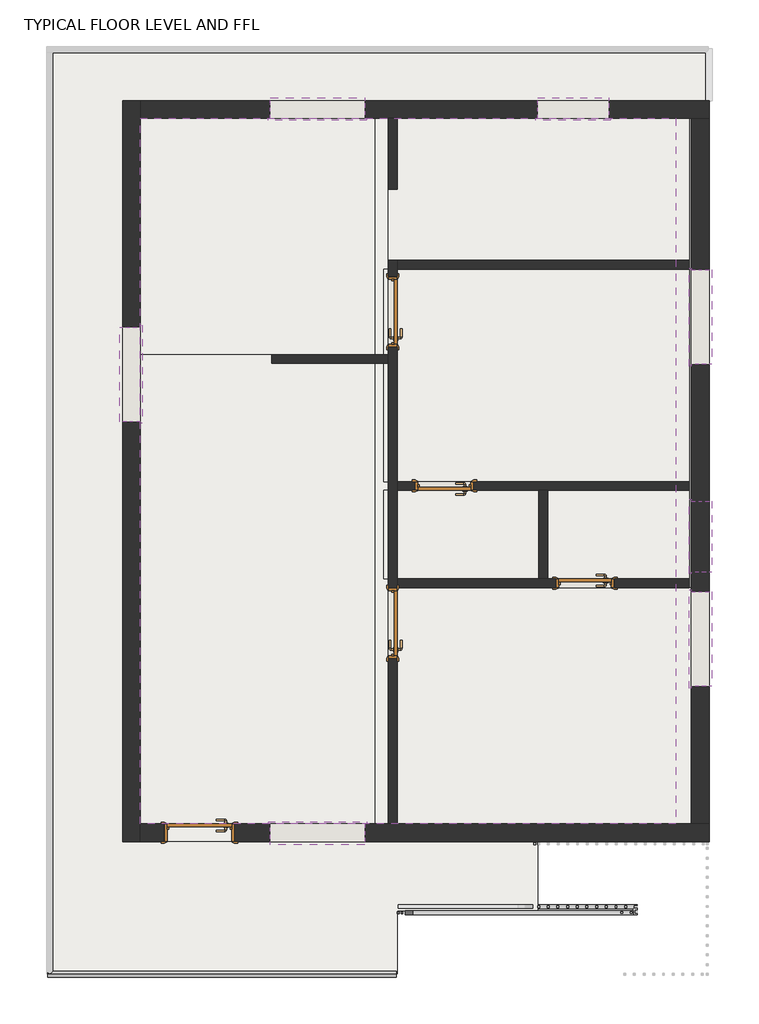
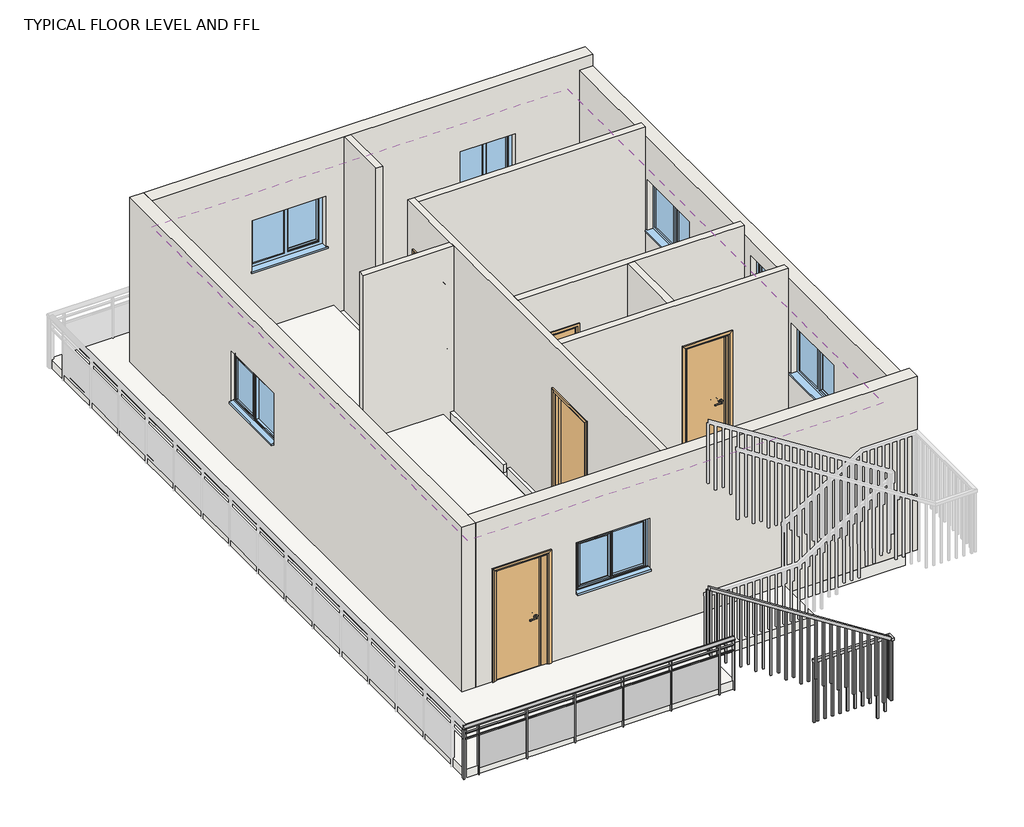
# One storey, part 1 of 3: 11 walls, 9 slabs, 7 windows, 5 doors, 2 railings, 1 covering.
"""IFC4 building model written with IfcOpenShell, lengths in millimetres."""

from ifc_helpers import new_model, si_unit, point, frame, origin, place, context, project, spatial, polyline, ellipse_curve, trimmed, outline, extrude, faceted_brep, transform, mapped, element, save
from ifc_brep_helpers import plane_surface, extruded_surface, advanced_brep
from components import doors_intsgl_d1_d2de26da, doors_intsgl_d1_5aeab8eb, doors_intsgl_d2_21b53886, doors_intsgl_d2_1f5f3f16, windows_dbl_plain_w1_9e0d93ab, windows_dbl_plain_w2_c69f14ef, windows_sgl_plain_v_28d0678b

model = new_model("IFC4")

# Units and contexts
model_context = context("Model", 3, world=origin())
ifc_project = project(units=[si_unit("LENGTHUNIT", "METRE", prefix="MILLI")], contexts=[model_context])

# Site, building, storey
site = spatial("IfcSite", under=ifc_project)
building = spatial("IfcBuilding", under=site)
storey = spatial("IfcBuildingStorey", under=building, Name="TYPICAL FLOOR LEVEL AND FFL", Elevation=3535.68)

# Covering
placement = place(None, origin())
element("IfcCovering", 1, at=placement, inside=storey, context=model_context, shape_type="SweptSolid", body=[
    extrude(outline(polyline([(-6897.0620435, -885.5593981), (-6897.0620435, -9991.0521308), (-10668.9827978, -9991.0521308), (-13810.6009005, -9991.0521308), (-13810.6009005, -885.5593981), (-6897.0620435, -885.5593981)])), frame((0.0, 0.0, 6126.48), z_axis=(0.0, 0.0, 1.0), x_axis=(1.0, 0.0, 0.0)), (0.0, 0.0, 1.0), 57.0),
])

# Doors
doors_intsgl_d1_shape = doors_intsgl_d1_d2de26da(model_context)
element("IfcDoor", 2, ObjectType="Doors_IntSgl : D1", at=placement, inside=storey, context=model_context, shape_type="MappedRepresentation", body=[
    mapped(doors_intsgl_d1_shape, transform((-10553.0840108, -7400.866169, 3685.6416), x_axis=(0.0, 1.0, 0.0), y_axis=(-1.0, 0.0, 0.0), z_axis=(0.0, 0.0, 1.0))),
])
element("IfcDoor", 3, ObjectType="Doors_IntSgl : D1", at=placement, inside=storey, context=model_context, shape_type="MappedRepresentation", body=[
    mapped(doors_intsgl_d1_shape, transform((-10553.0840108, -3381.2262014, 3685.6416), x_axis=(0.0, 1.0, 0.0), y_axis=(-1.0, 0.0, 0.0), z_axis=(0.0, 0.0, 1.0))),
])
doors_intsgl_d1_2_shape = doors_intsgl_d1_5aeab8eb(model_context)
element("IfcDoor", 4, ObjectType="Doors_IntSgl : D1", at=placement, inside=storey, context=model_context, shape_type="MappedRepresentation", body=[
    mapped(doors_intsgl_d1_2_shape, transform((-13048.4335145, -10105.3521308, 3535.68), x_axis=(-1.0, 0.0, 0.0), y_axis=(0.0, -1.0, 0.0), z_axis=(0.0, 0.0, 1.0))),
])
doors_intsgl_d2_shape = doors_intsgl_d2_21b53886(model_context)
element("IfcDoor", 5, ObjectType="Doors_IntSgl : D2", at=placement, inside=storey, context=model_context, shape_type="MappedRepresentation", body=[
    mapped(doors_intsgl_d2_shape, transform((-9886.3340108, -5628.9784114, 3685.6416), x_axis=(-1.0, 0.0, 0.0), y_axis=(0.0, -1.0, 0.0), z_axis=(0.0, 0.0, 1.0))),
])
doors_intsgl_d2_2_shape = doors_intsgl_d2_1f5f3f16(model_context)
element("IfcDoor", 6, ObjectType="Doors_IntSgl : D2", at=placement, inside=storey, context=model_context, shape_type="MappedRepresentation", body=[
    mapped(doors_intsgl_d2_2_shape, transform((-8070.4366309, -6886.516169, 3685.6416), x_axis=(-1.0, 0.0, 0.0), y_axis=(0.0, -1.0, 0.0), z_axis=(0.0, 0.0, 1.0))),
])

# Railings
element("IfcRailing", 7, ObjectType="1100mm", at=placement, inside=storey, context=model_context, shape_type="SolidModel", body=[
    faceted_brep([(-10457.8773536, -11114.0601959, 4838.88), (-10457.8773536, -11114.0601959, 4779.5164137), (-10457.8773536, -11164.0601959, 4779.5164137), (-10457.8773536, -11164.0601959, 4838.88), (-7447.5340108, -11114.0601959, 2912.2269781), (-7447.5340108, -11164.0601959, 2912.2269781), (-7447.5340108, -11164.0601959, 2852.8633918), (-7447.5340108, -11114.0601959, 2852.8633918)], [[[0, 1, 2, 3]], [[4, 5, 6, 7]], [[1, 0, 4, 7]], [[2, 1, 7, 6]], [[3, 2, 6, 5]], [[0, 3, 5, 4]]]),
    faceted_brep([(-7447.5340108, -11164.0601959, 2888.16), (-7447.5340108, -11164.0601959, 2838.16), (-7397.5340108, -11164.0601959, 2838.16), (-7397.5340108, -11164.0601959, 2888.16), (-7447.5340108, -11083.3255223, 2888.16), (-7447.5340108, -11083.3255223, 2838.16), (-7397.5340108, -11033.3255223, 2838.16), (-7397.5340108, -11033.3255223, 2888.16), (-8680.149573, -11083.3255223, 2888.16), (-8680.149573, -11033.3255223, 2888.16), (-8680.149573, -11033.3255223, 2838.16), (-8680.149573, -11083.3255223, 2838.16)], [[[0, 1, 2, 3]], [[1, 0, 4, 5]], [[2, 1, 5, 6]], [[3, 2, 6, 7]], [[0, 3, 7, 4]], [[8, 9, 10, 11]], [[5, 4, 8, 11]], [[6, 5, 11, 10]], [[7, 6, 10, 9]], [[4, 7, 9, 8]]]),
    extrude(outline(polyline([(-8597.5340108, -11045.8255223), (-8597.5340108, -11070.8255223), (-8622.5340108, -11070.8255223), (-8622.5340108, -11045.8255223), (-8597.5340108, -11045.8255223)])), frame((0.0, 0.0, 1788.16), z_axis=(0.0, 0.0, 1.0), x_axis=(1.0, 0.0, 0.0)), (0.0, 0.0, 1.0), 1050.0),
    extrude(outline(polyline([(-8472.5340108, -11045.8255223), (-8472.5340108, -11070.8255223), (-8497.5340108, -11070.8255223), (-8497.5340108, -11045.8255223), (-8472.5340108, -11045.8255223)])), frame((0.0, 0.0, 1788.16), z_axis=(0.0, 0.0, 1.0), x_axis=(1.0, 0.0, 0.0)), (0.0, 0.0, 1.0), 1050.0),
    extrude(outline(polyline([(-8347.5340108, -11045.8255223), (-8347.5340108, -11070.8255223), (-8372.5340108, -11070.8255223), (-8372.5340108, -11045.8255223), (-8347.5340108, -11045.8255223)])), frame((0.0, 0.0, 1788.16), z_axis=(0.0, 0.0, 1.0), x_axis=(1.0, 0.0, 0.0)), (0.0, 0.0, 1.0), 1050.0),
    extrude(outline(polyline([(-8222.5340108, -11045.8255223), (-8222.5340108, -11070.8255223), (-8247.5340108, -11070.8255223), (-8247.5340108, -11045.8255223), (-8222.5340108, -11045.8255223)])), frame((0.0, 0.0, 1788.16), z_axis=(0.0, 0.0, 1.0), x_axis=(1.0, 0.0, 0.0)), (0.0, 0.0, 1.0), 1050.0),
    extrude(outline(polyline([(-8097.5340108, -11045.8255223), (-8097.5340108, -11070.8255223), (-8122.5340108, -11070.8255223), (-8122.5340108, -11045.8255223), (-8097.5340108, -11045.8255223)])), frame((0.0, 0.0, 1788.16), z_axis=(0.0, 0.0, 1.0), x_axis=(1.0, 0.0, 0.0)), (0.0, 0.0, 1.0), 1050.0),
    extrude(outline(polyline([(-7972.5340108, -11045.8255223), (-7972.5340108, -11070.8255223), (-7997.5340108, -11070.8255223), (-7997.5340108, -11045.8255223), (-7972.5340108, -11045.8255223)])), frame((0.0, 0.0, 1788.16), z_axis=(0.0, 0.0, 1.0), x_axis=(1.0, 0.0, 0.0)), (0.0, 0.0, 1.0), 1050.0),
    extrude(outline(polyline([(-7847.5340108, -11045.8255223), (-7847.5340108, -11070.8255223), (-7872.5340108, -11070.8255223), (-7872.5340108, -11045.8255223), (-7847.5340108, -11045.8255223)])), frame((0.0, 0.0, 1788.16), z_axis=(0.0, 0.0, 1.0), x_axis=(1.0, 0.0, 0.0)), (0.0, 0.0, 1.0), 1050.0),
    extrude(outline(polyline([(-7722.5340108, -11045.8255223), (-7722.5340108, -11070.8255223), (-7747.5340108, -11070.8255223), (-7747.5340108, -11045.8255223), (-7722.5340108, -11045.8255223)])), frame((0.0, 0.0, 1788.16), z_axis=(0.0, 0.0, 1.0), x_axis=(1.0, 0.0, 0.0)), (0.0, 0.0, 1.0), 1050.0),
    extrude(outline(polyline([(-7597.5340108, -11045.8255223), (-7597.5340108, -11070.8255223), (-7622.5340108, -11070.8255223), (-7622.5340108, -11045.8255223), (-7597.5340108, -11045.8255223)])), frame((0.0, 0.0, 1484.4784954), z_axis=(0.0, 0.0, 1.0), x_axis=(1.0, 0.0, 0.0)), (0.0, 0.0, 1.0), 1353.6815046),
    extrude(outline(polyline([(-7472.5340108, -11045.8255223), (-7472.5340108, -11070.8255223), (-7497.5340108, -11070.8255223), (-7497.5340108, -11045.8255223), (-7472.5340108, -11045.8255223)])), frame((0.0, 0.0, 1564.4608651), z_axis=(0.0, 0.0, 1.0), x_axis=(1.0, 0.0, 0.0)), (0.0, 0.0, 1.0), 1273.6991349),
    extrude(outline(polyline([(-7410.0340108, -11089.0601959), (-7435.0340108, -11089.0601959), (-7435.0340108, -11064.0601959), (-7410.0340108, -11064.0601959), (-7410.0340108, -11089.0601959)])), frame((0.0, 0.0, 1770.6), z_axis=(0.0, 0.0, 1.0), x_axis=(1.0, 0.0, 0.0)), (0.0, 0.0, 1.0), 1067.56),
    extrude(outline(polyline([(2851.8393741, -7445.9340108), (1788.16, -7445.9340108), (1788.16, -7420.9340108), (2835.8390977, -7420.9340108), (2851.8393741, -7445.9340108)])), frame((0.0, -11151.5601959, 0.0), z_axis=(0.0, 1.0, 0.0), x_axis=(0.0, 0.0, 1.0)), (0.0, 0.0, 1.0), 25.0),
    extrude(outline(polyline([(2931.8407561, -7570.9340108), (1788.16, -7570.9340108), (1788.16, -7545.9340108), (2915.8404797, -7545.9340108), (2931.8407561, -7570.9340108)])), frame((0.0, -11151.5601959, 0.0), z_axis=(0.0, 1.0, 0.0), x_axis=(0.0, 0.0, 1.0)), (0.0, 0.0, 1.0), 25.0),
    extrude(outline(polyline([(3011.8421381, -7695.9340108), (1950.72, -7695.9340108), (1950.72, -7670.9340108), (2995.8418617, -7670.9340108), (3011.8421381, -7695.9340108)])), frame((0.0, -11151.5601959, 0.0), z_axis=(0.0, 1.0, 0.0), x_axis=(0.0, 0.0, 1.0)), (0.0, 0.0, 1.0), 25.0),
    extrude(outline(polyline([(3091.8435201, -7820.9340108), (1950.72, -7820.9340108), (1950.72, -7795.9340108), (3075.8432437, -7795.9340108), (3091.8435201, -7820.9340108)])), frame((0.0, -11151.5601959, 0.0), z_axis=(0.0, 1.0, 0.0), x_axis=(0.0, 0.0, 1.0)), (0.0, 0.0, 1.0), 25.0),
    extrude(outline(polyline([(3171.8449021, -7945.9340108), (2113.28, -7945.9340108), (2113.28, -7920.9340108), (3155.8446257, -7920.9340108), (3171.8449021, -7945.9340108)])), frame((0.0, -11151.5601959, 0.0), z_axis=(0.0, 1.0, 0.0), x_axis=(0.0, 0.0, 1.0)), (0.0, 0.0, 1.0), 25.0),
    extrude(outline(polyline([(3251.8462841, -8070.9340108), (2113.28, -8070.9340108), (2113.28, -8045.9340108), (3235.8460077, -8045.9340108), (3251.8462841, -8070.9340108)])), frame((0.0, -11151.5601959, 0.0), z_axis=(0.0, 1.0, 0.0), x_axis=(0.0, 0.0, 1.0)), (0.0, 0.0, 1.0), 25.0),
    extrude(outline(polyline([(3331.8476661, -8195.9340108), (2275.84, -8195.9340108), (2275.84, -8170.9340108), (3315.8473897, -8170.9340108), (3331.8476661, -8195.9340108)])), frame((0.0, -11151.5601959, 0.0), z_axis=(0.0, 1.0, 0.0), x_axis=(0.0, 0.0, 1.0)), (0.0, 0.0, 1.0), 25.0),
    extrude(outline(polyline([(3411.8490481, -8320.9340108), (2275.84, -8320.9340108), (2275.84, -8295.9340108), (3395.8487717, -8295.9340108), (3411.8490481, -8320.9340108)])), frame((0.0, -11151.5601959, 0.0), z_axis=(0.0, 1.0, 0.0), x_axis=(0.0, 0.0, 1.0)), (0.0, 0.0, 1.0), 25.0),
    extrude(outline(polyline([(3491.8504301, -8445.9340108), (2438.4, -8445.9340108), (2438.4, -8420.9340108), (3475.8501537, -8420.9340108), (3491.8504301, -8445.9340108)])), frame((0.0, -11151.5601959, 0.0), z_axis=(0.0, 1.0, 0.0), x_axis=(0.0, 0.0, 1.0)), (0.0, 0.0, 1.0), 25.0),
    extrude(outline(polyline([(3571.8518121, -8570.9340108), (2438.4, -8570.9340108), (2438.4, -8545.9340108), (3555.8515357, -8545.9340108), (3571.8518121, -8570.9340108)])), frame((0.0, -11151.5601959, 0.0), z_axis=(0.0, 1.0, 0.0), x_axis=(0.0, 0.0, 1.0)), (0.0, 0.0, 1.0), 25.0),
    extrude(outline(polyline([(3651.8531942, -8695.9340108), (2600.96, -8695.9340108), (2600.96, -8670.9340108), (3635.8529178, -8670.9340108), (3651.8531942, -8695.9340108)])), frame((0.0, -11151.5601959, 0.0), z_axis=(0.0, 1.0, 0.0), x_axis=(0.0, 0.0, 1.0)), (0.0, 0.0, 1.0), 25.0),
    extrude(outline(polyline([(3731.8545762, -8820.9340108), (2600.96, -8820.9340108), (2600.96, -8795.9340108), (3715.8542998, -8795.9340108), (3731.8545762, -8820.9340108)])), frame((0.0, -11151.5601959, 0.0), z_axis=(0.0, 1.0, 0.0), x_axis=(0.0, 0.0, 1.0)), (0.0, 0.0, 1.0), 25.0),
    extrude(outline(polyline([(3811.8559582, -8945.9340108), (2600.96, -8945.9340108), (2600.96, -8920.9340108), (3795.8556818, -8920.9340108), (3811.8559582, -8945.9340108)])), frame((0.0, -11151.5601959, 0.0), z_axis=(0.0, 1.0, 0.0), x_axis=(0.0, 0.0, 1.0)), (0.0, 0.0, 1.0), 25.0),
    extrude(outline(polyline([(3891.8573402, -9070.9340108), (2763.52, -9070.9340108), (2763.52, -9045.9340108), (3875.8570638, -9045.9340108), (3891.8573402, -9070.9340108)])), frame((0.0, -11151.5601959, 0.0), z_axis=(0.0, 1.0, 0.0), x_axis=(0.0, 0.0, 1.0)), (0.0, 0.0, 1.0), 25.0),
    extrude(outline(polyline([(3971.8587222, -9195.9340108), (2763.52, -9195.9340108), (2763.52, -9170.9340108), (3955.8584458, -9170.9340108), (3971.8587222, -9195.9340108)])), frame((0.0, -11151.5601959, 0.0), z_axis=(0.0, 1.0, 0.0), x_axis=(0.0, 0.0, 1.0)), (0.0, 0.0, 1.0), 25.0),
    extrude(outline(polyline([(4051.8601042, -9320.9340108), (2926.08, -9320.9340108), (2926.08, -9295.9340108), (4035.8598278, -9295.9340108), (4051.8601042, -9320.9340108)])), frame((0.0, -11151.5601959, 0.0), z_axis=(0.0, 1.0, 0.0), x_axis=(0.0, 0.0, 1.0)), (0.0, 0.0, 1.0), 25.0),
    extrude(outline(polyline([(4131.8614862, -9445.9340108), (2926.08, -9445.9340108), (2926.08, -9420.9340108), (4115.8612098, -9420.9340108), (4131.8614862, -9445.9340108)])), frame((0.0, -11151.5601959, 0.0), z_axis=(0.0, 1.0, 0.0), x_axis=(0.0, 0.0, 1.0)), (0.0, 0.0, 1.0), 25.0),
    extrude(outline(polyline([(4211.8628682, -9570.9340108), (3088.64, -9570.9340108), (3088.64, -9545.9340108), (4195.8625918, -9545.9340108), (4211.8628682, -9570.9340108)])), frame((0.0, -11151.5601959, 0.0), z_axis=(0.0, 1.0, 0.0), x_axis=(0.0, 0.0, 1.0)), (0.0, 0.0, 1.0), 25.0),
    extrude(outline(polyline([(4291.8642502, -9695.9340108), (3088.64, -9695.9340108), (3088.64, -9670.9340108), (4275.8639738, -9670.9340108), (4291.8642502, -9695.9340108)])), frame((0.0, -11151.5601959, 0.0), z_axis=(0.0, 1.0, 0.0), x_axis=(0.0, 0.0, 1.0)), (0.0, 0.0, 1.0), 25.0),
    extrude(outline(polyline([(4371.8656322, -9820.9340108), (3251.2, -9820.9340108), (3251.2, -9795.9340108), (4355.8653558, -9795.9340108), (4371.8656322, -9820.9340108)])), frame((0.0, -11151.5601959, 0.0), z_axis=(0.0, 1.0, 0.0), x_axis=(0.0, 0.0, 1.0)), (0.0, 0.0, 1.0), 25.0),
    extrude(outline(polyline([(4451.8670143, -9945.9340108), (3251.2, -9945.9340108), (3251.2, -9920.9340108), (4435.8667379, -9920.9340108), (4451.8670143, -9945.9340108)])), frame((0.0, -11151.5601959, 0.0), z_axis=(0.0, 1.0, 0.0), x_axis=(0.0, 0.0, 1.0)), (0.0, 0.0, 1.0), 25.0),
    extrude(outline(polyline([(4531.8683963, -10070.9340108), (3413.76, -10070.9340108), (3413.76, -10045.9340108), (4515.8681199, -10045.9340108), (4531.8683963, -10070.9340108)])), frame((0.0, -11151.5601959, 0.0), z_axis=(0.0, 1.0, 0.0), x_axis=(0.0, 0.0, 1.0)), (0.0, 0.0, 1.0), 25.0),
    extrude(outline(polyline([(4611.8697783, -10195.9340108), (3413.76, -10195.9340108), (3413.76, -10170.9340108), (4595.8695019, -10170.9340108), (4611.8697783, -10195.9340108)])), frame((0.0, -11151.5601959, 0.0), z_axis=(0.0, 1.0, 0.0), x_axis=(0.0, 0.0, 1.0)), (0.0, 0.0, 1.0), 25.0),
    extrude(outline(polyline([(4691.8711603, -10320.9340108), (3576.32, -10320.9340108), (3576.32, -10295.9340108), (4675.8708839, -10295.9340108), (4691.8711603, -10320.9340108)])), frame((0.0, -11151.5601959, 0.0), z_axis=(0.0, 1.0, 0.0), x_axis=(0.0, 0.0, 1.0)), (0.0, 0.0, 1.0), 25.0),
    extrude(outline(polyline([(4771.8725423, -10445.9340108), (3576.32, -10445.9340108), (3576.32, -10420.9340108), (4755.8722659, -10420.9340108), (4771.8725423, -10445.9340108)])), frame((0.0, -11151.5601959, 0.0), z_axis=(0.0, 1.0, 0.0), x_axis=(0.0, 0.0, 1.0)), (0.0, 0.0, 1.0), 25.0),
    extrude(outline(polyline([(-7410.0340108, -11070.8255223), (-7435.0340108, -11070.8255223), (-7435.0340108, -11045.8255223), (-7410.0340108, -11045.8255223), (-7410.0340108, -11070.8255223)])), frame((0.0, 0.0, 1770.6), z_axis=(0.0, 0.0, 1.0), x_axis=(1.0, 0.0, 0.0)), (0.0, 0.0, 1.0), 1067.56),
    extrude(outline(polyline([(2844.8632536, -7435.0340108), (1788.16, -7435.0340108), (1788.16, -7410.0340108), (2828.8629772, -7410.0340108), (2844.8632536, -7435.0340108)])), frame((0.0, -11151.5601959, 0.0), z_axis=(0.0, 1.0, 0.0), x_axis=(0.0, 0.0, 1.0)), (0.0, 0.0, 1.0), 25.0),
    extrude(outline(polyline([(-8655.149573, -11045.8255223), (-8655.149573, -11070.8255223), (-8680.149573, -11070.8255223), (-8680.149573, -11045.8255223), (-8655.149573, -11045.8255223)])), frame((0.0, 0.0, 1788.16), z_axis=(0.0, 0.0, 1.0), x_axis=(1.0, 0.0, 0.0)), (0.0, 0.0, 1.0), 1050.0),
    extrude(outline(polyline([(4803.8730951, -10495.9340108), (3738.88, -10495.9340108), (3738.88, -10470.9340108), (4787.8728187, -10470.9340108), (4803.8730951, -10495.9340108)])), frame((0.0, -11151.5601959, 0.0), z_axis=(0.0, 1.0, 0.0), x_axis=(0.0, 0.0, 1.0)), (0.0, 0.0, 1.0), 25.0),
])
element("IfcRailing", 8, ObjectType="Glass_Panel-Bottom_Fill", at=placement, inside=storey, context=model_context, shape_type="SolidModel", body=[
    advanced_brep(
    [(-15004.3420435, -11892.802126, 4435.68), (-15004.3420435, -11932.802126, 4405.68), (-15004.3420435, -11972.802126, 4435.68), (-15004.3420435, -11932.802126, 4465.68), (-10508.5420435, -11892.802126, 4435.68), (-10508.5420435, -11932.802126, 4465.68), (-10508.5420435, -11972.802126, 4435.68), (-10508.5420435, -11932.802126, 4405.68)],
    [
        (0, 1, ellipse_curve(frame((-15004.3420435, -11932.802126, 4435.68), z_axis=(-1.0, 0.0, 0.0), x_axis=(0.0, -1.0, 0.0)), 40.0, 30.0)),
        (1, 2, ellipse_curve(frame((-15004.3420435, -11932.802126, 4435.68), z_axis=(-1.0, 0.0, 0.0), x_axis=(0.0, -1.0, 0.0)), 40.0, 30.0)),
        (2, 3, ellipse_curve(frame((-15004.3420435, -11932.802126, 4435.68), z_axis=(-1.0, 0.0, 0.0), x_axis=(0.0, -1.0, 0.0)), 40.0, 30.0)),
        (3, 0, ellipse_curve(frame((-15004.3420435, -11932.802126, 4435.68), z_axis=(-1.0, 0.0, 0.0), x_axis=(0.0, -1.0, 0.0)), 40.0, 30.0)),
        (4, 5, ellipse_curve(frame((-10508.5420435, -11932.802126, 4435.68), z_axis=(1.0, 0.0, 0.0), x_axis=(0.0, -1.0, 0.0)), 40.0, 30.0)),
        (5, 6, ellipse_curve(frame((-10508.5420435, -11932.802126, 4435.68), z_axis=(1.0, 0.0, 0.0), x_axis=(0.0, -1.0, 0.0)), 40.0, 30.0)),
        (6, 7, ellipse_curve(frame((-10508.5420435, -11932.802126, 4435.68), z_axis=(1.0, 0.0, 0.0), x_axis=(0.0, -1.0, 0.0)), 40.0, 30.0)),
        (7, 4, ellipse_curve(frame((-10508.5420435, -11932.802126, 4435.68), z_axis=(1.0, 0.0, 0.0), x_axis=(0.0, -1.0, 0.0)), 40.0, 30.0)),
        (0, 4),
        (7, 1),
        (6, 2),
        (5, 3),
    ],
    [
        plane_surface(frame((-15004.3420435, -11932.802126, 4435.68), z_axis=(-1.0, 0.0, 0.0), x_axis=(0.0, 1.0, 0.0))),
        plane_surface(frame((-10508.5420435, -11932.802126, 4435.68), z_axis=(1.0, 0.0, 0.0), x_axis=(0.0, 1.0, 0.0))),
        extruded_surface(trimmed(ellipse_curve(frame((-10508.5420435, -11932.802126, 4435.68), z_axis=(-1.0, 0.0, 0.0), x_axis=(0.0, -1.0, 0.0)), 40.0, 30.0), [point((-10508.5420435, -11892.802126, 4435.68))], [point((-10508.5420435, -11932.802126, 4405.68))], True, "CARTESIAN"), (-4495.800000000001, 0.0, 0.0), 4495.800000000001),
        extruded_surface(trimmed(ellipse_curve(frame((-10508.5420435, -11932.802126, 4435.68), z_axis=(-1.0, 0.0, 0.0), x_axis=(0.0, -1.0, 0.0)), 40.0, 30.0), [point((-10508.5420435, -11932.802126, 4405.68))], [point((-10508.5420435, -11972.802126, 4435.68))], True, "CARTESIAN"), (-4495.800000000001, 0.0, 0.0), 4495.800000000001),
        extruded_surface(trimmed(ellipse_curve(frame((-10508.5420435, -11932.802126, 4435.68), z_axis=(-1.0, 0.0, 0.0), x_axis=(0.0, -1.0, 0.0)), 40.0, 30.0), [point((-10508.5420435, -11972.802126, 4435.68))], [point((-10508.5420435, -11932.802126, 4465.68))], True, "CARTESIAN"), (-4495.800000000001, 0.0, 0.0), 4495.800000000001),
        extruded_surface(trimmed(ellipse_curve(frame((-10508.5420435, -11932.802126, 4435.68), z_axis=(-1.0, 0.0, 0.0), x_axis=(0.0, -1.0, 0.0)), 40.0, 30.0), [point((-10508.5420435, -11932.802126, 4465.68))], [point((-10508.5420435, -11892.802126, 4435.68))], True, "CARTESIAN"), (-4495.800000000001, 0.0, 0.0), 4495.800000000001),
    ],
    [
        (0, [[1, 2, 3, 4]]),
        (1, [[5, 6, 7, 8]]),
        (2, [[-1, 9, -8, 10]]),
        (3, [[-2, -10, -7, 11]]),
        (4, [[-3, -11, -6, 12]]),
        (5, [[-4, -12, -5, -9]]),
    ],
),
    extrude(outline(polyline([(-15004.3420435, -11942.1928911), (-15004.3420435, -11922.1928911), (-10508.5420435, -11922.1928911), (-10508.5420435, -11942.1928911), (-15004.3420435, -11942.1928911)])), frame((0.0, 0.0, 4315.68), z_axis=(0.0, 0.0, 1.0), x_axis=(1.0, 0.0, 0.0)), (0.0, 0.0, 1.0), 20.0),
    extrude(outline(polyline([(-15004.3420435, -11942.1928911), (-15004.3420435, -11922.1928911), (-10508.5420435, -11922.1928911), (-10508.5420435, -11942.1928911), (-15004.3420435, -11942.1928911)])), frame((0.0, 0.0, 4215.68), z_axis=(0.0, 0.0, 1.0), x_axis=(1.0, 0.0, 0.0)), (0.0, 0.0, 1.0), 20.0),
    extrude(outline(polyline([(-10762.4420435, -11907.1928911), (-10750.4420435, -11907.1928911), (-10750.4420435, -11957.1928911), (-10762.4420435, -11957.1928911), (-10762.4420435, -11907.1928911)])), frame((0.0, 0.0, 3535.68), z_axis=(0.0, 0.0, 1.0), x_axis=(1.0, 0.0, 0.0)), (0.0, 0.0, 1.0), 870.0),
    extrude(outline(polyline([(-11556.4420435, -11933.9177012), (-10756.4420435, -11933.9177012), (-10756.4420435, -11938.9177012), (-11556.4420435, -11938.9177012), (-11556.4420435, -11933.9177012)])), frame((0.0, 0.0, 3635.68), z_axis=(0.0, 0.0, 1.0), x_axis=(1.0, 0.0, 0.0)), (0.0, 0.0, 1.0), 600.0),
    extrude(outline(polyline([(-11562.4420435, -11907.1928911), (-11550.4420435, -11907.1928911), (-11550.4420435, -11957.1928911), (-11562.4420435, -11957.1928911), (-11562.4420435, -11907.1928911)])), frame((0.0, 0.0, 3535.68), z_axis=(0.0, 0.0, 1.0), x_axis=(1.0, 0.0, 0.0)), (0.0, 0.0, 1.0), 870.0),
    extrude(outline(polyline([(-12356.4420435, -11933.9177012), (-11556.4420435, -11933.9177012), (-11556.4420435, -11938.9177012), (-12356.4420435, -11938.9177012), (-12356.4420435, -11933.9177012)])), frame((0.0, 0.0, 3635.68), z_axis=(0.0, 0.0, 1.0), x_axis=(1.0, 0.0, 0.0)), (0.0, 0.0, 1.0), 600.0),
    extrude(outline(polyline([(-12362.4420435, -11907.1928911), (-12350.4420435, -11907.1928911), (-12350.4420435, -11957.1928911), (-12362.4420435, -11957.1928911), (-12362.4420435, -11907.1928911)])), frame((0.0, 0.0, 3535.68), z_axis=(0.0, 0.0, 1.0), x_axis=(1.0, 0.0, 0.0)), (0.0, 0.0, 1.0), 870.0),
    extrude(outline(polyline([(-13156.4420435, -11933.9177012), (-12356.4420435, -11933.9177012), (-12356.4420435, -11938.9177012), (-13156.4420435, -11938.9177012), (-13156.4420435, -11933.9177012)])), frame((0.0, 0.0, 3635.68), z_axis=(0.0, 0.0, 1.0), x_axis=(1.0, 0.0, 0.0)), (0.0, 0.0, 1.0), 600.0),
    extrude(outline(polyline([(-13162.4420435, -11907.1928911), (-13150.4420435, -11907.1928911), (-13150.4420435, -11957.1928911), (-13162.4420435, -11957.1928911), (-13162.4420435, -11907.1928911)])), frame((0.0, 0.0, 3535.68), z_axis=(0.0, 0.0, 1.0), x_axis=(1.0, 0.0, 0.0)), (0.0, 0.0, 1.0), 870.0),
    extrude(outline(polyline([(-13956.4420435, -11933.9177012), (-13156.4420435, -11933.9177012), (-13156.4420435, -11938.9177012), (-13956.4420435, -11938.9177012), (-13956.4420435, -11933.9177012)])), frame((0.0, 0.0, 3635.68), z_axis=(0.0, 0.0, 1.0), x_axis=(1.0, 0.0, 0.0)), (0.0, 0.0, 1.0), 600.0),
    extrude(outline(polyline([(-13962.4420435, -11907.1928911), (-13950.4420435, -11907.1928911), (-13950.4420435, -11957.1928911), (-13962.4420435, -11957.1928911), (-13962.4420435, -11907.1928911)])), frame((0.0, 0.0, 3535.68), z_axis=(0.0, 0.0, 1.0), x_axis=(1.0, 0.0, 0.0)), (0.0, 0.0, 1.0), 870.0),
    extrude(outline(polyline([(-14756.4420435, -11933.9177012), (-13956.4420435, -11933.9177012), (-13956.4420435, -11938.9177012), (-14756.4420435, -11938.9177012), (-14756.4420435, -11933.9177012)])), frame((0.0, 0.0, 3635.68), z_axis=(0.0, 0.0, 1.0), x_axis=(1.0, 0.0, 0.0)), (0.0, 0.0, 1.0), 600.0),
    extrude(outline(polyline([(-14762.4420435, -11907.1928911), (-14750.4420435, -11907.1928911), (-14750.4420435, -11957.1928911), (-14762.4420435, -11957.1928911), (-14762.4420435, -11907.1928911)])), frame((0.0, 0.0, 3535.68), z_axis=(0.0, 0.0, 1.0), x_axis=(1.0, 0.0, 0.0)), (0.0, 0.0, 1.0), 870.0),
    extrude(outline(polyline([(-10516.5420435, -11907.1928911), (-10504.5420435, -11907.1928911), (-10504.5420435, -11957.1928911), (-10516.5420435, -11957.1928911), (-10516.5420435, -11907.1928911)])), frame((0.0, 0.0, 3535.68), z_axis=(0.0, 0.0, 1.0), x_axis=(1.0, 0.0, 0.0)), (0.0, 0.0, 1.0), 870.0),
    extrude(outline(polyline([(-15008.3420435, -11907.1928911), (-14996.3420435, -11907.1928911), (-14996.3420435, -11957.1928911), (-15008.3420435, -11957.1928911), (-15008.3420435, -11907.1928911)])), frame((0.0, 0.0, 3535.68), z_axis=(0.0, 0.0, 1.0), x_axis=(1.0, 0.0, 0.0)), (0.0, 0.0, 1.0), 870.0),
])

# Slabs
element("IfcSlab", 9, ObjectType="BATHROOM FLOORING", at=placement, inside=storey, context=model_context, shape_type="SweptSolid", body=[
    extrude(outline(polyline([(-8667.3366309, -5686.1284114), (-8667.3366309, -6829.366169), (-10668.9827978, -6829.366169), (-10668.9827978, -5686.1284114), (-8667.3366309, -5686.1284114)])), frame((0.0, 0.0, 3535.68), z_axis=(0.0, 0.0, 1.0), x_axis=(1.0, 0.0, 0.0)), (0.0, 0.0, 1.0), 149.9616),
])
element("IfcSlab", 10, ObjectType="BATHROOM FLOORING", at=placement, inside=storey, context=model_context, shape_type="SweptSolid", body=[
    extrude(outline(polyline([(-6724.371003, -5686.0601635), (-6724.371003, -6829.366169), (-8553.0366309, -6829.366169), (-8553.0366309, -5686.0601635), (-6724.371003, -5686.0601635)])), frame((0.0, 0.0, 3535.68), z_axis=(0.0, 0.0, 1.0), x_axis=(1.0, 0.0, 0.0)), (0.0, 0.0, 1.0), 149.9616),
])
element("IfcSlab", 11, ObjectType="BED ROOM FLOORING", at=placement, inside=storey, context=model_context, shape_type="SweptSolid", body=[
    extrude(outline(polyline([(-6724.371003, -2828.9136626), (-6724.371003, -5571.8284114), (-10668.9827978, -5571.8284114), (-10668.9827978, -2828.9136626), (-6724.371003, -2828.9136626)])), frame((0.0, 0.0, 3535.68), z_axis=(0.0, 0.0, 1.0), x_axis=(1.0, 0.0, 0.0)), (0.0, 0.0, 1.0), 149.9616),
])
element("IfcSlab", 12, ObjectType="BED ROOM FLOORING", at=placement, inside=storey, context=model_context, shape_type="SweptSolid", body=[
    extrude(outline(polyline([(-6698.6395131, -6943.5979211), (-6698.6395131, -9991.1886267), (-10495.9340108, -9991.1886267), (-10495.9340108, -6943.5979211), (-6698.6395131, -6943.5979211)])), frame((0.0, 0.0, 3535.68), z_axis=(0.0, 0.0, 1.0), x_axis=(1.0, 0.0, 0.0)), (0.0, 0.0, 1.0), 149.9616),
])
element("IfcSlab", 13, ObjectType="DINING FLOORING", at=placement, inside=storey, context=model_context, shape_type="SweptSolid", body=[
    extrude(outline(polyline([(-10783.2827978, -885.9480347), (-10783.2827978, -3933.5387403), (-13810.6009005, -3933.5387403), (-13810.6009005, -885.9480347), (-10783.2827978, -885.9480347)])), frame((0.0, 0.0, 3535.68), z_axis=(0.0, 0.0, 1.0), x_axis=(1.0, 0.0, 0.0)), (0.0, 0.0, 1.0), 149.9616),
])
element("IfcSlab", 14, ObjectType="HALL FLOORING", at=placement, inside=storey, context=model_context, shape_type="SweptSolid", body=[
    extrude(outline(polyline([(-10783.2827978, -3933.5387403), (-10783.2827978, -9991.0521308), (-13810.6009005, -9991.0521308), (-13810.6009005, -3933.5387403), (-10783.2827978, -3933.5387403)])), frame((0.0, 0.0, 3535.68), z_axis=(0.0, 0.0, 1.0), x_axis=(1.0, 0.0, 0.0)), (0.0, 0.0, 1.0), 149.9616),
])
element("IfcSlab", 15, ObjectType="KITCHEN FLOOR", at=placement, inside=storey, context=model_context, shape_type="SweptSolid", body=[
    extrude(outline(polyline([(-6724.371003, -885.9480347), (-6724.371003, -2714.6136626), (-10610.2340108, -2714.6136626), (-10610.2340108, -1800.3480347), (-10495.9340108, -1800.3480347), (-10495.9340108, -885.9480347), (-6724.371003, -885.9480347)])), frame((0.0, 0.0, 3535.68), z_axis=(0.0, 0.0, 1.0), x_axis=(1.0, 0.0, 0.0)), (0.0, 0.0, 1.0), 149.9616),
])
element("IfcSlab", 16, ObjectType="OUTER FLOORING", at=placement, inside=storey, context=model_context, shape_type="SweptSolid", body=[
    extrude(outline(polyline([(-14979.3420435, -11928.1928911), (-14979.3420435, 3.4571089), (-6470.371003, 3.4571089), (-6470.371003, -656.9593981), (-6495.4132565, -656.9593981), (-14039.0335145, -656.9593981), (-14039.0335145, -10219.6521308), (-8680.149573, -10219.6521308), (-8680.149573, -11109.5255223), (-10495.9340108, -11109.5255223), (-10495.9340108, -11928.1928911), (-14979.3420435, -11928.1928911)])), frame((0.0, 0.0, 3535.68), z_axis=(0.0, 0.0, 1.0), x_axis=(1.0, 0.0, 0.0)), (0.0, 0.0, 1.0), 149.9616),
])
element("IfcSlab", 17, ObjectType="RCC SLAB", at=placement, inside=storey, context=model_context, shape_type="Brep", body=[
    faceted_brep([(-6668.4620435, -656.9593981, 3335.7312), (-6668.4620435, -885.5593981, 3335.7312), (-6668.4620435, -10219.6521308, 3335.7312), (-6897.0620435, -10219.6521308, 3335.7312), (-10783.2827978, -10219.6521308, 3335.7312), (-14039.0335145, -10219.6521308, 3335.7312), (-14039.0335145, -885.5593981, 3335.7312), (-14039.0335145, -656.9593981, 3335.7312), (-6668.4620435, -656.9593981, 3535.68), (-14039.0335145, -656.9593981, 3535.68), (-14039.0335145, -885.5593981, 3535.68), (-14039.0335145, -10219.6521308, 3535.68), (-6668.4620435, -10219.6521308, 3535.68)], [[[0, 1, 2, 3, 4, 5, 6, 7]], [[8, 9, 10, 11, 12]], [[2, 1, 0, 8, 12]], [[5, 4, 3, 2, 12, 11]], [[7, 6, 5, 11, 10, 9]], [[0, 7, 9, 8]]]),
])

# Walls
element("IfcWall", 18, ObjectType="EXT WALL", at=placement, inside=storey, context=model_context, shape_type="Brep", body=[
    faceted_brep([(-14039.0335145, -656.9593981, 3535.68), (-14039.0335145, -10219.6521308, 3535.68), (-14039.0335145, -10219.6521308, 6583.68), (-14039.0335145, -656.9593981, 6583.68), (-14039.0335145, -4797.1593981, 5645.68), (-14039.0335145, -4797.1593981, 4735.68), (-14039.0335145, -3577.9593981, 4735.68), (-14039.0335145, -3577.9593981, 5645.68), (-13810.4335145, -656.9593981, 3535.68), (-13810.4335145, -656.9593981, 6583.68), (-13810.4335145, -885.5593981, 6583.68), (-13810.4335145, -9991.0521308, 6583.68), (-13810.4335145, -10219.6521308, 6583.68), (-13810.4335145, -10219.6521308, 3535.68), (-13810.4335145, -9991.0521308, 3535.68), (-13810.4335145, -885.5593981, 3535.68), (-13810.4335145, -4797.1593981, 5645.68), (-13810.4335145, -3577.9593981, 5645.68), (-13810.4335145, -3577.9593981, 4735.68), (-13810.4335145, -4797.1593981, 4735.68)], [[[0, 1, 2, 3], [4, 5, 6, 7]], [[8, 9, 10, 11, 12, 13, 14, 15], [16, 17, 18, 19]], [[1, 0, 8, 15, 14, 13]], [[3, 2, 12, 11, 10, 9]], [[2, 1, 13, 12]], [[0, 3, 9, 8]], [[5, 4, 16, 19]], [[6, 5, 19, 18]], [[7, 6, 18, 17]], [[4, 7, 17, 16]]]),
])
element("IfcWall", 19, ObjectType="EXT WALL", at=placement, inside=storey, context=model_context, shape_type="Brep", body=[
    faceted_brep([(-13810.4335145, -9991.0521308, 6583.68), (-10610.2340108, -9991.0521308, 6583.68), (-10495.9340108, -9991.0521308, 6583.68), (-6470.371003, -9991.0521308, 6583.68), (-6470.371003, -9991.0521308, 6383.7312), (-6470.371003, -9991.0521308, 3535.68), (-6698.971003, -9991.0521308, 3535.68), (-10495.9340108, -9991.0521308, 3535.68), (-10610.2340108, -9991.0521308, 3535.68), (-12591.2335145, -9991.0521308, 3535.68), (-12591.2335145, -9991.0521308, 5645.68), (-13505.6335145, -9991.0521308, 5645.68), (-13505.6335145, -9991.0521308, 3535.68), (-13810.4335145, -9991.0521308, 3535.68), (-10915.0340108, -9991.0521308, 5645.68), (-12134.2340108, -9991.0521308, 5645.68), (-12134.2340108, -9991.0521308, 4735.68), (-10915.0340108, -9991.0521308, 4735.68), (-6470.371003, -10219.6521308, 6583.68), (-13810.4335145, -10219.6521308, 6583.68), (-13810.4335145, -10219.6521308, 3535.68), (-13505.6335145, -10219.6521308, 3535.68), (-13505.6335145, -10219.6521308, 5645.68), (-12591.2335145, -10219.6521308, 5645.68), (-12591.2335145, -10219.6521308, 3535.68), (-6470.371003, -10219.6521308, 3535.68), (-10915.0340108, -10219.6521308, 5645.68), (-10915.0340108, -10219.6521308, 4735.68), (-12134.2340108, -10219.6521308, 4735.68), (-12134.2340108, -10219.6521308, 5645.68)], [[[0, 1, 2, 3, 4, 5, 6, 7, 8, 9, 10, 11, 12, 13], [14, 15, 16, 17]], [[18, 19, 20, 21, 22, 23, 24, 25], [26, 27, 28, 29]], [[20, 13, 12, 21]], [[5, 25, 24, 9, 8, 7, 6]], [[3, 2, 1, 0, 19, 18]], [[0, 13, 20, 19]], [[5, 4, 3, 18, 25]], [[11, 22, 21, 12]], [[22, 11, 10, 23]], [[23, 10, 9, 24]], [[27, 26, 14, 17]], [[28, 27, 17, 16]], [[29, 28, 16, 15]], [[26, 29, 15, 14]]]),
])
element("IfcWall", 20, ObjectType="EXT WALL", at=placement, inside=storey, context=model_context, shape_type="Brep", body=[
    faceted_brep([(-13810.4335145, -885.5593981, 3535.68), (-6698.971003, -885.5593981, 3535.68), (-6470.371003, -885.5593981, 3535.68), (-6470.371003, -885.5593981, 6383.7312), (-6470.371003, -885.5593981, 6583.68), (-13810.4335145, -885.5593981, 6583.68), (-8679.8132565, -885.5593981, 5645.68), (-7765.4132565, -885.5593981, 5645.68), (-7765.4132565, -885.5593981, 4735.68), (-8679.8132565, -885.5593981, 4735.68), (-12134.0335145, -885.5593981, 5645.68), (-10914.8335145, -885.5593981, 5645.68), (-10914.8335145, -885.5593981, 4735.68), (-12134.0335145, -885.5593981, 4735.68), (-13810.4335145, -656.9593981, 3535.68), (-13810.4335145, -656.9593981, 6583.68), (-6470.371003, -656.9593981, 6583.68), (-6470.371003, -656.9593981, 3535.68), (-8679.8132565, -656.9593981, 5645.68), (-8679.8132565, -656.9593981, 4735.68), (-7765.4132565, -656.9593981, 4735.68), (-7765.4132565, -656.9593981, 5645.68), (-12134.0335145, -656.9593981, 5645.68), (-12134.0335145, -656.9593981, 4735.68), (-10914.8335145, -656.9593981, 4735.68), (-10914.8335145, -656.9593981, 5645.68)], [[[0, 1, 2, 3, 4, 5], [6, 7, 8, 9], [10, 11, 12, 13]], [[14, 15, 16, 17], [18, 19, 20, 21], [22, 23, 24, 25]], [[2, 1, 0, 14, 17]], [[5, 4, 16, 15]], [[0, 5, 15, 14]], [[4, 3, 2, 17, 16]], [[19, 18, 6, 9]], [[20, 19, 9, 8]], [[21, 20, 8, 7]], [[18, 21, 7, 6]], [[23, 22, 10, 13]], [[24, 23, 13, 12]], [[25, 24, 12, 11]], [[22, 25, 11, 10]]]),
])
element("IfcWall", 21, ObjectType="EXT WALL", at=placement, inside=storey, context=model_context, shape_type="SweptSolid", body=[
    extrude(outline(polyline([(-885.5593981, 3535.68), (-9991.0521308, 3535.68), (-9991.0521308, 6383.7312), (-885.5593981, 6383.7312), (-885.5593981, 3535.68)]), holes=[polyline([(-5825.4521308, 6122.08), (-6739.8521308, 6122.08), (-6739.8521308, 5212.08), (-5825.4521308, 5212.08), (-5825.4521308, 6122.08)]), polyline([(-2841.3593981, 5645.68), (-4060.5593981, 5645.68), (-4060.5593981, 4735.68), (-2841.3593981, 4735.68), (-2841.3593981, 5645.68)]), polyline([(-6993.8521308, 5645.68), (-8213.0521308, 5645.68), (-8213.0521308, 4735.68), (-6993.8521308, 4735.68), (-6993.8521308, 5645.68)])]), frame((-6698.971003, 0.0, 0.0), z_axis=(1.0, 0.0, 0.0), x_axis=(0.0, 1.0, 0.0)), (0.0, 0.0, 1.0), 228.6),
])
element("IfcWall", 22, ObjectType="INT WALL", at=placement, inside=storey, context=model_context, shape_type="SweptSolid", body=[
    extrude(outline(polyline([(-10610.2340108, -1800.3480347), (-10610.2340108, -885.9480347), (-10495.9340108, -885.9480347), (-10495.9340108, -1800.3480347), (-10610.2340108, -1800.3480347)])), frame((0.0, 0.0, 3535.68), z_axis=(0.0, 0.0, 1.0), x_axis=(1.0, 0.0, 0.0)), (0.0, 0.0, 1.0), 3048.0),
])
element("IfcWall", 23, ObjectType="INT WALL", at=placement, inside=storey, context=model_context, shape_type="SweptSolid", body=[
    extrude(outline(polyline([(-10495.9340108, -2714.6136626), (-6724.371003, -2714.6136626), (-6724.371003, -2828.9136626), (-10495.9340108, -2828.9136626), (-10495.9340108, -2714.6136626)])), frame((0.0, 0.0, 3535.68), z_axis=(0.0, 0.0, 1.0), x_axis=(1.0, 0.0, 0.0)), (0.0, 0.0, 1.0), 3048.0),
])
element("IfcWall", 24, ObjectType="INT WALL", at=placement, inside=storey, context=model_context, shape_type="Brep", body=[
    faceted_brep([(-10495.9340108, -5686.1284114, 3535.68), (-8667.3366309, -5686.1284114, 3535.68), (-8553.0366309, -5686.1284114, 3535.68), (-6724.371003, -5686.1284114, 3535.68), (-6724.371003, -5686.1284114, 6583.68), (-8553.0366309, -5686.1284114, 6583.68), (-8667.3366309, -5686.1284114, 6583.68), (-10495.9340108, -5686.1284114, 6583.68), (-10267.3340108, -5686.1284114, 3685.6416), (-10267.3340108, -5686.1284114, 5795.6416), (-9505.3340108, -5686.1284114, 5795.6416), (-9505.3340108, -5686.1284114, 3685.6416), (-6724.371003, -5571.8284114, 3535.68), (-10495.9340108, -5571.8284114, 3535.68), (-10495.9340108, -5571.8284114, 6583.68), (-6724.371003, -5571.8284114, 6583.68), (-10267.3340108, -5571.8284114, 5795.6416), (-10267.3340108, -5571.8284114, 3685.6416), (-9505.3340108, -5571.8284114, 3685.6416), (-9505.3340108, -5571.8284114, 5795.6416)], [[[0, 1, 2, 3, 4, 5, 6, 7], [8, 9, 10, 11]], [[12, 13, 14, 15], [16, 17, 18, 19]], [[3, 2, 1, 0, 13, 12]], [[4, 3, 12, 15]], [[7, 6, 5, 4, 15, 14]], [[0, 7, 14, 13]], [[8, 17, 16, 9]], [[9, 16, 19, 10]], [[10, 19, 18, 11]], [[17, 8, 11, 18]]]),
])
element("IfcWall", 25, ObjectType="INT WALL", at=placement, inside=storey, context=model_context, shape_type="Brep", body=[
    faceted_brep([(-10495.9340108, -6943.666169, 3539.0136234), (-6724.371003, -6943.666169, 3539.0136234), (-6724.371003, -6943.666169, 6583.68), (-10495.9340108, -6943.666169, 6583.68), (-8451.4366309, -6943.666169, 3685.6416), (-8451.4366309, -6943.666169, 5795.6416), (-7689.4366309, -6943.666169, 5795.6416), (-7689.4366309, -6943.666169, 3685.6416), (-6724.371003, -6829.366169, 3539.0136234), (-10495.9340108, -6829.366169, 3539.0136234), (-10495.9340108, -6829.366169, 6583.68), (-8667.3366309, -6829.366169, 6583.68), (-8553.0366309, -6829.366169, 6583.68), (-6724.371003, -6829.366169, 6583.68), (-8451.4366309, -6829.366169, 5795.6416), (-8451.4366309, -6829.366169, 3685.6416), (-7689.4366309, -6829.366169, 3685.6416), (-7689.4366309, -6829.366169, 5795.6416)], [[[0, 1, 2, 3], [4, 5, 6, 7]], [[8, 9, 10, 11, 12, 13], [14, 15, 16, 17]], [[1, 0, 9, 8]], [[2, 1, 8, 13]], [[3, 2, 13, 12, 11, 10]], [[0, 3, 10, 9]], [[4, 15, 14, 5]], [[5, 14, 17, 6]], [[6, 17, 16, 7]], [[15, 4, 7, 16]]]),
])
element("IfcWall", 26, ObjectType="INT WALL", at=placement, inside=storey, context=model_context, shape_type="SweptSolid", body=[
    extrude(outline(polyline([(-8667.3366309, -6829.366169), (-8667.3366309, -5686.1284114), (-8553.0366309, -5686.1284114), (-8553.0366309, -6829.366169), (-8667.3366309, -6829.366169)])), frame((0.0, 0.0, 3535.68), z_axis=(0.0, 0.0, 1.0), x_axis=(1.0, 0.0, 0.0)), (0.0, 0.0, 1.0), 3048.0),
])
element("IfcWall", 27, ObjectType="INT WALL", at=placement, inside=storey, context=model_context, shape_type="SweptSolid", body=[
    extrude(outline(polyline([(-10610.2340108, -4047.8387403), (-12112.7859221, -4047.8387403), (-12112.7859221, -3933.5387403), (-10610.2340108, -3933.5387403), (-10610.2340108, -4047.8387403)])), frame((0.0, 0.0, 3535.68), z_axis=(0.0, 0.0, 1.0), x_axis=(1.0, 0.0, 0.0)), (0.0, 0.0, 1.0), 3048.0),
])
element("IfcWall", 28, ObjectType="INT WALL", at=placement, inside=storey, context=model_context, shape_type="Brep", body=[
    faceted_brep([(-10610.2340108, -2714.6136626, 3535.68), (-10610.2340108, -3933.5387403, 3535.68), (-10610.2340108, -4047.8387403, 3535.68), (-10610.2340108, -9991.0521308, 3535.68), (-10610.2340108, -9991.0521308, 6583.68), (-10610.2340108, -4047.8387403, 6583.68), (-10610.2340108, -3933.5387403, 6583.68), (-10610.2340108, -2714.6136626, 6583.68), (-10610.2340108, -6943.666169, 3685.6416), (-10610.2340108, -6943.666169, 5795.6416), (-10610.2340108, -7858.066169, 5795.6416), (-10610.2340108, -7858.066169, 3685.6416), (-10610.2340108, -2924.0262014, 3685.6416), (-10610.2340108, -2924.0262014, 5795.6416), (-10610.2340108, -3838.4262014, 5795.6416), (-10610.2340108, -3838.4262014, 3685.6416), (-10495.9340108, -2714.6136626, 3535.68), (-10495.9340108, -2714.6136626, 6583.68), (-10495.9340108, -2828.9136626, 6583.68), (-10495.9340108, -5571.8284114, 6583.68), (-10495.9340108, -5686.1284114, 6583.68), (-10495.9340108, -6829.366169, 6583.68), (-10495.9340108, -6943.666169, 6583.68), (-10495.9340108, -9991.0521308, 6583.68), (-10495.9340108, -9991.0521308, 3535.68), (-10495.9340108, -5686.1284114, 3535.68), (-10495.9340108, -5571.8284114, 3535.68), (-10495.9340108, -2828.9136626, 3535.68), (-10495.9340108, -6943.666169, 3685.6416), (-10495.9340108, -7858.066169, 3685.6416), (-10495.9340108, -7858.066169, 5795.6416), (-10495.9340108, -6943.666169, 5795.6416), (-10495.9340108, -2924.0262014, 3685.6416), (-10495.9340108, -3838.4262014, 3685.6416), (-10495.9340108, -3838.4262014, 5795.6416), (-10495.9340108, -2924.0262014, 5795.6416)], [[[0, 1, 2, 3, 4, 5, 6, 7], [8, 9, 10, 11], [12, 13, 14, 15]], [[16, 17, 18, 19, 20, 21, 22, 23, 24, 25, 26, 27], [28, 29, 30, 31], [32, 33, 34, 35]], [[3, 2, 1, 0, 16, 27, 26, 25, 24]], [[7, 6, 5, 4, 23, 22, 21, 20, 19, 18, 17]], [[0, 7, 17, 16]], [[4, 3, 24, 23]], [[8, 11, 29, 28]], [[11, 10, 30, 29]], [[10, 9, 31, 30]], [[9, 8, 28, 31]], [[12, 15, 33, 32]], [[15, 14, 34, 33]], [[14, 13, 35, 34]], [[13, 12, 32, 35]]]),
])

# Windows
windows_dbl_plain_w1_shape = windows_dbl_plain_w1_9e0d93ab(model_context)
element("IfcWindow", 29, ObjectType="Windows_Dbl_Plain : W1", at=placement, inside=storey, context=model_context, shape_type="MappedRepresentation", body=[
    mapped(windows_dbl_plain_w1_shape, transform((-6593.1275708, -7888.4521308, 3535.68), x_axis=(0.0, -1.0, 0.0), y_axis=(1.0, 0.0, 0.0), z_axis=(0.0, 0.0, 1.0))),
])
element("IfcWindow", 30, ObjectType="Windows_Dbl_Plain : W1", at=placement, inside=storey, context=model_context, shape_type="MappedRepresentation", body=[
    mapped(windows_dbl_plain_w1_shape, transform((-6593.1275708, -3735.9593981, 3535.68), x_axis=(0.0, -1.0, 0.0), y_axis=(1.0, 0.0, 0.0), z_axis=(0.0, 0.0, 1.0))),
])
element("IfcWindow", 31, ObjectType="Windows_Dbl_Plain : W1", at=placement, inside=storey, context=model_context, shape_type="MappedRepresentation", body=[
    mapped(windows_dbl_plain_w1_shape, transform((-11239.4335145, -779.7159659, 3535.68), x_axis=(1.0, 0.0, 0.0), y_axis=(0.0, 1.0, 0.0), z_axis=(0.0, 0.0, 1.0))),
])
element("IfcWindow", 32, ObjectType="Windows_Dbl_Plain : W1", at=placement, inside=storey, context=model_context, shape_type="MappedRepresentation", body=[
    mapped(windows_dbl_plain_w1_shape, transform((-13916.2769467, -3902.5593981, 3535.68), x_axis=(0.0, 1.0, 0.0), y_axis=(-1.0, 0.0, 0.0), z_axis=(0.0, 0.0, 1.0))),
])
element("IfcWindow", 33, ObjectType="Windows_Dbl_Plain : W1", at=placement, inside=storey, context=model_context, shape_type="MappedRepresentation", body=[
    mapped(windows_dbl_plain_w1_shape, transform((-11809.6340108, -10096.895563, 3535.68), x_axis=(-1.0, 0.0, 0.0), y_axis=(0.0, -1.0, 0.0), z_axis=(0.0, 0.0, 1.0))),
])
windows_dbl_plain_w2_shape = windows_dbl_plain_w2_c69f14ef(model_context)
element("IfcWindow", 34, ObjectType="Windows_Dbl_Plain : W2", at=placement, inside=storey, context=model_context, shape_type="MappedRepresentation", body=[
    mapped(windows_dbl_plain_w2_shape, transform((-7937.6132565, -779.7159659, 3535.68), x_axis=(1.0, 0.0, 0.0), y_axis=(0.0, 1.0, 0.0), z_axis=(0.0, 0.0, 1.0))),
])
windows_sgl_plain_v_shape = windows_sgl_plain_v_28d0678b(model_context)
element("IfcWindow", 35, ObjectType="Windows_Sgl_Plain : V", at=placement, inside=storey, context=model_context, shape_type="MappedRepresentation", body=[
    mapped(windows_sgl_plain_v_shape, transform((-6593.1275708, -6282.6521308, 4012.08), x_axis=(0.0, -1.0, 0.0), y_axis=(1.0, 0.0, 0.0), z_axis=(0.0, 0.0, 1.0))),
])

save(model, "model.ifc")

# Revit data of these elements
# Type
#   Keynote = "K40"
#   built-in parameter 1002203 = 1 (stored number, unit not read)
#   built-in parameter 1002202 = 1 (stored number, unit not read)
#   Layers, outside or top first: 0.147638 ft "Metal Stud Layer" (function 1); 0.03937 ft "Gypsum Wall Board" (function 1)
# Type "Doors_IntSgl : D1"
#   Type Mark = "46"
#   Type Comments = "Internal Single"
#   Operation = "SingleSwingRight"
#   Manufacturer = "Revit"
#   Keynote = "L20"
#   Description = "Internal Single Door"
#   Analytic Construction = "Metal"
#   UnderCut = 0.026247 ft
#   Tolerance = 0.006562 ft
#   Thickness = 0.124672 ft
#   Thermal Resistance (R) = 0.270117 (m²·K)/W
#   Structural Tolerance = 0.026247 ft
#   StopDepth = 0.104987 ft
#   Stop Thickness = 0.062336 ft
#   Rough Width = 3.0 ft
#   Rough Height = 6.922572 ft
#   Height to Top Lock Rail = 3.28084 ft
#   Heat Transfer Coefficient (U) = 3.7021 W/(m²·K)
#   Handle Z Distance = 2.952756 ft
#   Handle X Distance = 0.246063 ft
#   Frame Thickness = 0.104987 ft
#   Door Panel Width = 2.724409 ft
#   Door Panel Thickness = 0.124672 ft
#   Door Panel Offset = 0.0 ft
#   Height = 6.922572 ft
#   Width = 3.0 ft
#   Door Panel Height = 6.75853 ft
#   Architrave Setback = 0.016404 ft
#   Vis - Ironmongery = yes
#   Material Ironmongery = Door - Handle
#   Material Frame = Door - Frame/Mullion (1)
#   Material Door = Door - Panel
#   Material Architrave = Door - Architrave
#   Visual Light Transmittance = 0
#   Solar Heat Gain Coefficient = 0
#   Function = (empty or 0)
#   Wall Closure = (empty or 0)
# Type "Doors_IntSgl : D2"
#   Type Mark = "47"
#   Type Comments = "Internal Single"
#   Operation = "SingleSwingRight"
#   Manufacturer = "Revit"
#   Keynote = "L20"
#   Description = "Internal Single Door"
#   Analytic Construction = "Metal"
#   UnderCut = 0.026247 ft
#   Tolerance = 0.006562 ft
#   Thickness = 0.124672 ft
#   Thermal Resistance (R) = 0.270117 (m²·K)/W
#   Structural Tolerance = 0.026247 ft
#   StopDepth = 0.104987 ft
#   Stop Thickness = 0.062336 ft
#   Rough Width = 2.5 ft
#   Rough Height = 6.922572 ft
#   Height to Top Lock Rail = 3.28084 ft
#   Heat Transfer Coefficient (U) = 3.7021 W/(m²·K)
#   Handle Z Distance = 2.952756 ft
#   Handle X Distance = 0.246063 ft
#   Frame Thickness = 0.104987 ft
#   Door Panel Width = 2.224409 ft
#   Door Panel Thickness = 0.124672 ft
#   Door Panel Offset = 0.0 ft
#   Height = 6.922572 ft
#   Width = 2.5 ft
#   Door Panel Height = 6.75853 ft
#   Architrave Setback = 0.016404 ft
#   Vis - Ironmongery = yes
#   Material Ironmongery = Door - Handle
#   Material Frame = Door - Frame/Mullion (1)
#   Material Door = Door - Panel
#   Material Architrave = Door - Architrave
#   Visual Light Transmittance = 0
#   Solar Heat Gain Coefficient = 0
#   Function = (empty or 0)
#   Wall Closure = (empty or 0)
# Type "1100mm"
#   built-in parameter 1008612 = 0.019685 (stored number, unit not read)
#   built-in parameter 1008611 = 0.019685 (stored number, unit not read)
#   built-in parameter 1008609 = 0.902231 (stored number, unit not read)
#   built-in parameter 1008604 = 0.19685 (stored number, unit not read)
#   built-in parameter 1008603 = 0.164042 (stored number, unit not read)
#   Railing Height = 3.608924 ft
#   built-in parameter 1008630 = 2
#   built-in parameter 1008610 = 2
#   built-in parameter 1008608 = 1
#   built-in parameter 1008618 = Baluster_Square : 25mm
# Type "Glass_Panel-Bottom_Fill"
#   built-in parameter 1008612 = 0.019685 (stored number, unit not read)
#   built-in parameter 1008611 = 0.019685 (stored number, unit not read)
#   built-in parameter 1008609 = 0.902231 (stored number, unit not read)
#   built-in parameter 1008604 = 0.19685 (stored number, unit not read)
#   built-in parameter 1008603 = 0.164042 (stored number, unit not read)
#   Railing Height = 2.952756 ft
#   built-in parameter 1008630 = 2
#   built-in parameter 1008610 = 2
# Type "BATHROOM FLOORING"
#   Function = 0
#   Layers, outside or top first: 0.072 ft "BATHROOM FLOOR" (function 5); 0.42 ft "Structure, Timber Joist/Rafter Layer" (function 1)
# Type "BED ROOM FLOORING"
#   Function = 0
#   Layers, outside or top first: 0.072 ft "BEDROOM FLOOR" (function 5); 0.42 ft "Structure, Timber Joist/Rafter Layer" (function 1)
# Type "DINING FLOORING"
#   Function = 0
#   Layers, outside or top first: 0.072 ft "KITCHEN FLOOR" (function 5); 0.42 ft "Structure, Timber Joist/Rafter Layer" (function 1)
# Type "HALL FLOORING"
#   Function = 0
#   Layers, outside or top first: 0.072 ft "HALL FLOOR" (function 5); 0.42 ft "Structure, Timber Joist/Rafter Layer" (function 1)
# Type "KITCHEN FLOOR"
#   Function = 0
#   Layers, outside or top first: 0.072 ft "KITCHEN FLOOR" (function 5); 0.42 ft "Structure, Timber Joist/Rafter Layer" (function 1)
# Type "OUTER FLOORING"
#   Function = 0
#   Layers, outside or top first: 0.072 ft "Concrete Masonry Units _High Density" (function 5); 0.42 ft "Structure, Timber Joist/Rafter Layer" (function 1)
# Type "RCC SLAB"
#   Layers, outside or top first: 0.656 ft no material (function 1)
# Type "EXT WALL"
#   Keynote = "F10"
#   Layers, outside or top first: 0.75 ft "Brick, Common" (function 1)
# Type "INT WALL"
#   Keynote = "F10"
#   Layers, outside or top first: 0.375 ft "Brick, Common" (function 1)
# Type "Windows_Dbl_Plain : W1"
#   Type Mark = "56"
#   Operation = "DoublePanelVertical"
#   Construction Type Id = "GSP4R"
#   Manufacturer = "Revit"
#   Keynote = "L10"
#   Analytic Construction = "1/8 in Pilkington single glazing"
#   Wrap Layers (Ext) from Ext = 0.336286 ft
#   Wrap Layers (Int) from Ext = 0.582349 ft
#   Window Board Projection = 0.082021 ft
#   Window Board Extension = 0.082021 ft
#   Visual Light Transmittance = 0.9
#   Solar Heat Gain Coefficient = 0.78
#   Rough Width = 4.0 ft
#   Rough Height = 2.985564 ft
#   Height = 2.985564 ft
#   Width = 4.0 ft
#   Heat Transfer Coefficient (U) = 3.6886 W/(m²·K)
#   Glazing Thickness = 0.07874 ft
#   FrameOffset - External = 0.164042 ft
#   Frame Depth = 0.213255 ft
#   Default Head Height = 6.922572 ft
#   Cill Depth = 0.287073 ft
#   Cavity Closer Width = 0.164042 ft
#   Cavity Closer Offset from Ext = 0.336286 ft
#   Cavity Closer Depth = 0.278871 ft
#   Vis - Cavity Closers = yes
#   Define Thermal Properties by = 1
#   Material Trim = Window Frame
#   Material Glass = Glass
#   Material Frame = Window Frame
#   Wall Closure = (empty or 0)
# Type "Windows_Dbl_Plain : W2"
#   Type Mark = "57"
#   Operation = "DoublePanelVertical"
#   Construction Type Id = "GSP4R"
#   Manufacturer = "Revit"
#   Keynote = "L10"
#   Analytic Construction = "1/8 in Pilkington single glazing"
#   Wrap Layers (Ext) from Ext = 0.336286 ft
#   Wrap Layers (Int) from Ext = 0.582349 ft
#   Window Board Projection = 0.082021 ft
#   Window Board Extension = 0.082021 ft
#   Visual Light Transmittance = 0.9
#   Solar Heat Gain Coefficient = 0.78
#   Rough Width = 3.0 ft
#   Rough Height = 2.985564 ft
#   Height = 2.985564 ft
#   Width = 3.0 ft
#   Heat Transfer Coefficient (U) = 3.6886 W/(m²·K)
#   Glazing Thickness = 0.07874 ft
#   FrameOffset - External = 0.164042 ft
#   Frame Depth = 0.213255 ft
#   Default Head Height = 6.922572 ft
#   Cill Depth = 0.287073 ft
#   Cavity Closer Width = 0.164042 ft
#   Cavity Closer Offset from Ext = 0.336286 ft
#   Cavity Closer Depth = 0.278871 ft
#   Vis - Cavity Closers = yes
#   Define Thermal Properties by = 1
#   Material Trim = Window Frame
#   Material Glass = Glass
#   Material Frame = Window Frame
#   Wall Closure = (empty or 0)
# Type "Windows_Sgl_Plain : V"
#   Type Mark = "58"
#   Operation = "SinglePanel"
#   Construction Type Id = "SGL"
#   Manufacturer = "Revit"
#   Keynote = "L10"
#   Analytic Construction = "Large single-glazed windows"
#   Wrap Layers (Ext) from Ext = 0.336286 ft
#   Wrap Layers (Int) from Ext = 0.582349 ft
#   Window Board Projection = 0.082021 ft
#   Window Board Extension = 0.082021 ft
#   Visual Light Transmittance = 0.9
#   Solar Heat Gain Coefficient = 0.86
#   Rough Width = 3.0 ft
#   Rough Height = 2.985564 ft
#   Height = 2.985564 ft
#   Width = 3.0 ft
#   Heat Transfer Coefficient (U) = 5.5617 W/(m²·K)
#   Glazing Thickness = 0.07874 ft
#   FrameOffset - External = 0.164042 ft
#   Frame Depth = 0.213255 ft
#   Default Head Height = 6.922572 ft
#   Cill Depth = 0.287073 ft
#   Cavity Closer Width = 0.164042 ft
#   Cavity Closer Offset from Ext = 0.336286 ft
#   Cavity Closer Depth = 0.278871 ft
#   Vis - Cavity Closers = yes
#   Define Thermal Properties by = 1
#   Material Trim = Window Frame
#   Material Glass = Glass
#   Material Frame = Window Frame
#   Wall Closure = (empty or 0)
# Element 1 (IfcCovering)
#   Height Offset From Level = 8.5 ft
#   Phase Created = New Construction
#   Materials on its faces: "Gypsum Wall Board", "Metal Stud Layer"
# Elements 2, 3, 4 (IfcDoor, "Doors_IntSgl : D1")
#   Phase Created = New Construction
